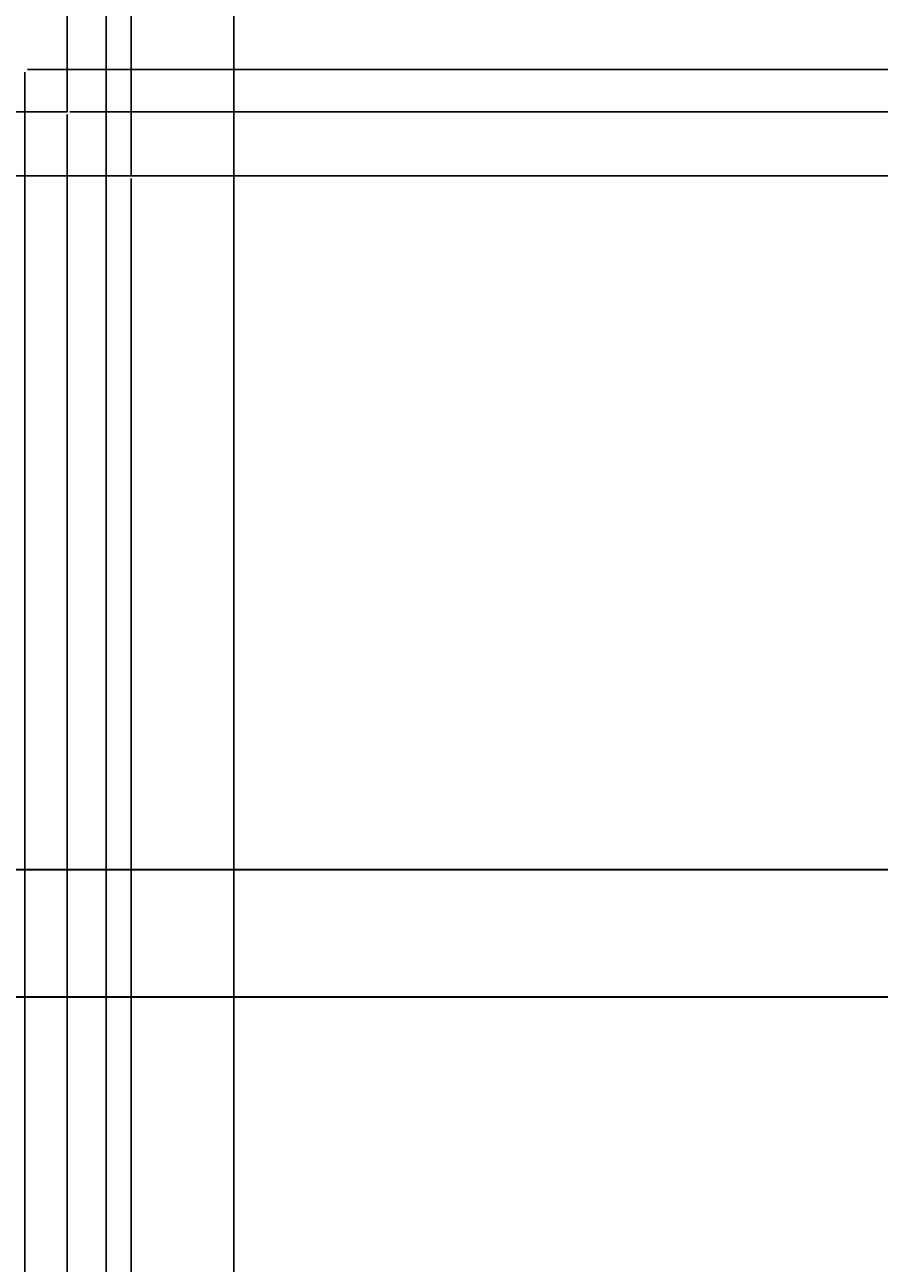
# Model space of a CAD drawing. Units: inches. Extents: x -6 to 289, y -8 to 323.
# Tile 55 of 107: x 166 to 186, y 153 to 182. Entities that reach past the tile are written whole.
import ezdxf

# ---------------------------------------------------------------- set-up
doc = ezdxf.new("R2010")
doc.units = ezdxf.units.IN
doc.header["$MEASUREMENT"] = 0
for name, color, linetype, lineweight in [('A-ANNO-DIMS', 2, 'Continuous', 18), ('A-ELEV', 7, 'Continuous', 35), ('A-GLAZ', 4, 'Continuous', 25)]:
    doc.layers.add(name, color=color, linetype=linetype, lineweight=lineweight)
doc.styles.get("Standard").update_dxf_attribs({"font": 'arial.ttf'})
doc.dimstyles.get("Standard").update_dxf_attribs({"dimtxt": 0.18, "dimasz": 0.18, "dimexe": 0.18, "dimexo": 0.0625, "dimgap": 0.09, "dimtad": 0, "dimtih": 1, "dimtoh": 1, "dimdec": 4, "dimzin": 0, "dimdsep": 46, "dimtxsty": 'Standard', "dimcen": 0.09, "dimadec": 0, "dimazin": 0, "dimtfac": 1, "dimtdec": 4, "dimtofl": 0, "dimtmove": 0, "dimatfit": 3, "dimfxl": 1, "dimtolj": 1, "dimtzin": 0, "dimarcsym": 0})

# ---------------------------------------------------------------- blocks, each defined once
blk = doc.blocks.new('*U4')
for p, q in [((40.5, 46.5), (40.5, 1.5)), ((40.5, 1.5), (21, 1.5))]:
    blk.add_line(p, q)
blk.add_lwpolyline([(0, 0), (0, 48), (42, 48), (42, 0)], close=True)
blk = doc.blocks.new('*D24')
at = {"layer": 'A-ANNO-DIMS', "color": 0, "lineweight": -2, "transparency": 16777216}
for p, q in [((126.946, 178.654), (288.653, 178.654)), ((288.473, 178.474), (288.473, 159.153)), ((288.473, 139.469), (288.473, 158.789)), ((259.226, 139.289), (288.653, 139.289))]:
    blk.add_line(p, q, dxfattribs=at)
at = {"layer": 'A-ANNO-DIMS', "color": 0, "transparency": 16777216}
for points in [[(288.443, 178.474), (288.503, 178.474), (288.473, 178.654)], [(288.443, 139.469), (288.503, 139.469), (288.473, 139.289)]]:
    blk.add_solid(points, dxfattribs=at)
at = {"layer": 'Defpoints', "color": 0, "transparency": 16777216}
for p in [(126.883, 178.654), (288.473, 178.654), (259.164, 139.289)]:
    blk.add_point(p, dxfattribs=at)
at = {"layer": 'A-ANNO-DIMS', "color": 0, "transparency": 16777216, "insert": (288.473, 158.971), "char_height": 0.18, "attachment_point": 5}
blk.add_mtext('\\A1;39.365', dxfattribs=at)
blk = doc.blocks.new('*D25')
at = {"layer": 'A-ANNO-DIMS', "color": 0, "lineweight": -2, "transparency": 16777216}
for p, q in [((126.946, 226.654), (288.653, 226.654)), ((288.473, 226.474), (288.473, 202.836)), ((288.473, 178.834), (288.473, 202.472)), ((126.946, 178.654), (288.653, 178.654))]:
    blk.add_line(p, q, dxfattribs=at)
at = {"layer": 'A-ANNO-DIMS', "color": 0, "transparency": 16777216}
for points in [[(288.443, 226.474), (288.503, 226.474), (288.473, 226.654)], [(288.443, 178.834), (288.503, 178.834), (288.473, 178.654)]]:
    blk.add_solid(points, dxfattribs=at)
at = {"layer": 'Defpoints', "color": 0, "transparency": 16777216}
for p in [(126.883, 226.654), (288.473, 226.654), (126.883, 178.654)]:
    blk.add_point(p, dxfattribs=at)
at = {"layer": 'A-ANNO-DIMS', "color": 0, "transparency": 16777216, "insert": (288.473, 202.654), "char_height": 0.18, "attachment_point": 5}
blk.add_mtext('\\A1;48', dxfattribs=at)
blk = doc.blocks.new('*D32')
at = {"layer": 'A-ANNO-DIMS', "color": 0, "lineweight": -2, "transparency": 16777216}
for p, q in [((147.883, 181.092), (147.883, -8.391)), ((166.383, 181.092), (166.383, -8.391)), ((148.063, -8.211), (156.817, -8.211)), ((166.203, -8.211), (157.449, -8.211))]:
    blk.add_line(p, q, dxfattribs=at)
at = {"layer": 'A-ANNO-DIMS', "color": 0, "transparency": 16777216}
for points in [[(148.063, -8.181), (148.063, -8.241), (147.883, -8.211)], [(166.203, -8.181), (166.203, -8.241), (166.383, -8.211)]]:
    blk.add_solid(points, dxfattribs=at)
at = {"layer": 'Defpoints', "color": 0, "transparency": 16777216}
for p in [(147.883, 181.154), (166.383, 181.154), (166.383, -8.211)]:
    blk.add_point(p, dxfattribs=at)
at = {"layer": 'A-ANNO-DIMS', "color": 0, "transparency": 16777216, "insert": (157.133, -8.211), "char_height": 0.18, "attachment_point": 5}
blk.add_mtext('\\A1;18.5', dxfattribs=at)
blk = doc.blocks.new('*D33')
at = {"layer": 'A-ANNO-DIMS', "color": 0, "lineweight": -2, "transparency": 16777216}
for p, q in [((166.383, 181.092), (166.383, -8.391)), ((167.383, 180.092), (167.383, -8.391)), ((166.563, -8.211), (166.76, -8.211)), ((167.203, -8.211), (167.007, -8.211))]:
    blk.add_line(p, q, dxfattribs=at)
at = {"layer": 'A-ANNO-DIMS', "color": 0, "transparency": 16777216}
for points in [[(166.563, -8.181), (166.563, -8.241), (166.383, -8.211)], [(167.203, -8.181), (167.203, -8.241), (167.383, -8.211)]]:
    blk.add_solid(points, dxfattribs=at)
at = {"layer": 'Defpoints', "color": 0, "transparency": 16777216}
for p in [(166.383, 181.154), (167.383, 180.154), (167.383, -8.211)]:
    blk.add_point(p, dxfattribs=at)
at = {"layer": 'A-ANNO-DIMS', "color": 0, "transparency": 16777216, "insert": (166.883, -8.211), "char_height": 0.18, "attachment_point": 5}
blk.add_mtext('\\A1;1', dxfattribs=at)
blk = doc.blocks.new('*D34')
at = {"layer": 'A-ANNO-DIMS', "color": 0, "lineweight": -2, "transparency": 16777216}
for p, q in [((167.383, 180.092), (167.383, -8.391)), ((168.883, 178.592), (168.883, -8.391)), ((167.563, -8.211), (167.887, -8.211)), ((168.703, -8.211), (168.38, -8.211))]:
    blk.add_line(p, q, dxfattribs=at)
at = {"layer": 'A-ANNO-DIMS', "color": 0, "transparency": 16777216}
for points in [[(167.563, -8.181), (167.563, -8.241), (167.383, -8.211)], [(168.703, -8.181), (168.703, -8.241), (168.883, -8.211)]]:
    blk.add_solid(points, dxfattribs=at)
at = {"layer": 'Defpoints', "color": 0, "transparency": 16777216}
for p in [(167.383, 180.154), (168.883, 178.654), (168.883, -8.211)]:
    blk.add_point(p, dxfattribs=at)
at = {"layer": 'A-ANNO-DIMS', "color": 0, "transparency": 16777216, "insert": (168.133, -8.211), "char_height": 0.18, "attachment_point": 5}
blk.add_mtext('\\A1;1.5', dxfattribs=at)
blk = doc.blocks.new('*D35')
at = {"layer": 'A-ANNO-DIMS', "color": 0, "lineweight": -2, "transparency": 16777216}
for p, q in [((167.446, 180.154), (288.653, 180.154)), ((288.473, 179.974), (288.473, 179.586)), ((288.473, 178.834), (288.473, 179.222)), ((168.946, 178.654), (288.653, 178.654))]:
    blk.add_line(p, q, dxfattribs=at)
at = {"layer": 'A-ANNO-DIMS', "color": 0, "transparency": 16777216}
for points in [[(288.443, 179.974), (288.503, 179.974), (288.473, 180.154)], [(288.443, 178.834), (288.503, 178.834), (288.473, 178.654)]]:
    blk.add_solid(points, dxfattribs=at)
at = {"layer": 'Defpoints', "color": 0, "transparency": 16777216}
for p in [(167.383, 180.154), (288.473, 180.154), (168.883, 178.654)]:
    blk.add_point(p, dxfattribs=at)
at = {"layer": 'A-ANNO-DIMS', "color": 0, "transparency": 16777216, "insert": (288.473, 179.404), "char_height": 0.18, "attachment_point": 5}
blk.add_mtext('\\A1;1.5', dxfattribs=at)
blk = doc.blocks.new('*D36')
at = {"layer": 'A-ANNO-DIMS', "color": 0, "lineweight": -2, "transparency": 16777216}
for p, q in [((166.446, 181.154), (288.653, 181.154)), ((288.473, 180.974), (288.473, 180.834)), ((288.473, 180.334), (288.473, 180.474)), ((167.446, 180.154), (288.653, 180.154))]:
    blk.add_line(p, q, dxfattribs=at)
at = {"layer": 'A-ANNO-DIMS', "color": 0, "transparency": 16777216}
for points in [[(288.443, 180.974), (288.503, 180.974), (288.473, 181.154)], [(288.443, 180.334), (288.503, 180.334), (288.473, 180.154)]]:
    blk.add_solid(points, dxfattribs=at)
at = {"layer": 'Defpoints', "color": 0, "transparency": 16777216}
for p in [(166.383, 181.154), (288.473, 181.154), (167.383, 180.154)]:
    blk.add_point(p, dxfattribs=at)
at = {"layer": 'A-ANNO-DIMS', "color": 0, "transparency": 16777216, "insert": (288.473, 180.654), "char_height": 0.18, "attachment_point": 5}
blk.add_mtext('\\A1;1', dxfattribs=at)
blk = doc.blocks.new('*D37')
at = {"layer": 'A-ANNO-DIMS', "color": 0, "lineweight": -2, "transparency": 16777216}
for p, q in [((166.446, 224.154), (288.653, 224.154)), ((288.473, 223.974), (288.473, 202.836)), ((288.473, 181.334), (288.473, 202.472)), ((166.446, 181.154), (288.653, 181.154))]:
    blk.add_line(p, q, dxfattribs=at)
at = {"layer": 'A-ANNO-DIMS', "color": 0, "transparency": 16777216}
for points in [[(288.443, 223.974), (288.503, 223.974), (288.473, 224.154)], [(288.443, 181.334), (288.503, 181.334), (288.473, 181.154)]]:
    blk.add_solid(points, dxfattribs=at)
at = {"layer": 'Defpoints', "color": 0, "transparency": 16777216}
for p in [(166.383, 224.154), (288.473, 224.154), (166.383, 181.154)]:
    blk.add_point(p, dxfattribs=at)
at = {"layer": 'A-ANNO-DIMS', "color": 0, "transparency": 16777216, "insert": (288.473, 202.654), "char_height": 0.18, "attachment_point": 5}
blk.add_mtext('\\A1;43', dxfattribs=at)
blk = doc.blocks.new('*D77')
at = {"layer": 'A-ANNO-DIMS', "color": 0, "lineweight": -2, "transparency": 16777216}
for p, q in [((164.296, 51.148), (164.296, 322.969)), ((168.296, 51.148), (168.296, 322.969)), ((164.476, 322.789), (166.144, 322.789)), ((168.116, 322.789), (166.448, 322.789))]:
    blk.add_line(p, q, dxfattribs=at)
at = {"layer": 'A-ANNO-DIMS', "color": 0, "transparency": 16777216}
for points in [[(164.476, 322.819), (164.476, 322.759), (164.296, 322.789)], [(168.116, 322.819), (168.116, 322.759), (168.296, 322.789)]]:
    blk.add_solid(points, dxfattribs=at)
at = {"layer": 'Defpoints', "color": 0, "transparency": 16777216}
for p in [(168.296, 322.789), (164.296, 51.085), (168.296, 51.085)]:
    blk.add_point(p, dxfattribs=at)
at = {"layer": 'A-ANNO-DIMS', "color": 0, "transparency": 16777216, "insert": (166.296, 322.789), "char_height": 0.18, "attachment_point": 5}
blk.add_mtext('\\A1;4', dxfattribs=at)
blk = doc.blocks.new('*D78')
at = {"layer": 'A-ANNO-DIMS', "color": 0, "lineweight": -2, "transparency": 16777216}
for p, q in [((168.296, 51.148), (168.296, 322.969)), ((171.296, 51.148), (171.296, 322.969)), ((168.476, 322.789), (169.647, 322.789)), ((171.116, 322.789), (169.945, 322.789))]:
    blk.add_line(p, q, dxfattribs=at)
at = {"layer": 'A-ANNO-DIMS', "color": 0, "transparency": 16777216}
for points in [[(168.476, 322.819), (168.476, 322.759), (168.296, 322.789)], [(171.116, 322.819), (171.116, 322.759), (171.296, 322.789)]]:
    blk.add_solid(points, dxfattribs=at)
at = {"layer": 'Defpoints', "color": 0, "transparency": 16777216}
for p in [(171.296, 322.789), (168.296, 51.085), (171.296, 51.085)]:
    blk.add_point(p, dxfattribs=at)
at = {"layer": 'A-ANNO-DIMS', "color": 0, "transparency": 16777216, "insert": (169.796, 322.789), "char_height": 0.18, "attachment_point": 5}
blk.add_mtext('\\A1;3', dxfattribs=at)
blk = doc.blocks.new('*D79')
at = {"layer": 'A-ANNO-DIMS', "color": 0, "lineweight": -2, "transparency": 16777216}
for p, q in [((171.296, 118.033), (171.296, 322.969)), ((188.292, 116.842), (188.292, 322.969)), ((171.476, 322.789), (179.339, 322.789)), ((188.112, 322.789), (180.249, 322.789))]:
    blk.add_line(p, q, dxfattribs=at)
at = {"layer": 'A-ANNO-DIMS', "color": 0, "transparency": 16777216}
for points in [[(171.476, 322.819), (171.476, 322.759), (171.296, 322.789)], [(188.112, 322.819), (188.112, 322.759), (188.292, 322.789)]]:
    blk.add_solid(points, dxfattribs=at)
at = {"layer": 'Defpoints', "color": 0, "transparency": 16777216}
for p in [(188.292, 322.789), (171.296, 117.971), (188.292, 116.779)]:
    blk.add_point(p, dxfattribs=at)
at = {"layer": 'A-ANNO-DIMS', "color": 0, "transparency": 16777216, "insert": (179.794, 322.789), "char_height": 0.18, "attachment_point": 5}
blk.add_mtext('\\A1;16.996', dxfattribs=at)
blk = doc.blocks.new('*D96')
at = {"layer": 'A-ANNO-DIMS', "color": 0, "lineweight": -2, "transparency": 16777216}
for p, q in [((164.004, 159.411), (164.004, 322.969)), ((200.616, 159.411), (200.616, 322.969)), ((164.184, 322.789), (181.934, 322.789)), ((200.436, 322.789), (182.686, 322.789))]:
    blk.add_line(p, q, dxfattribs=at)
at = {"layer": 'A-ANNO-DIMS', "color": 0, "transparency": 16777216}
for points in [[(164.184, 322.819), (164.184, 322.759), (164.004, 322.789)], [(200.436, 322.819), (200.436, 322.759), (200.616, 322.789)]]:
    blk.add_solid(points, dxfattribs=at)
at = {"layer": 'Defpoints', "color": 0, "transparency": 16777216}
for p in [(200.616, 322.789), (164.004, 159.348), (200.616, 159.348)]:
    blk.add_point(p, dxfattribs=at)
at = {"layer": 'A-ANNO-DIMS', "color": 0, "transparency": 16777216, "insert": (182.31, 322.789), "char_height": 0.18, "attachment_point": 5}
blk.add_mtext('\\A1;36.61', dxfattribs=at)

msp = doc.modelspace()

# ---------------------------------------------------------------- linework, layer by layer
at = {"layer": 'A-ELEV'}
for points in [[(247.1638, 139.2888), (115.1638, 139.2888), (115.1638, 162.3484), (247.1638, 162.3484)], [(244.1638, 142.2888), (118.1638, 142.2888), (118.1638, 159.3484), (244.1638, 159.3484)]]:
    msp.add_lwpolyline(points, close=True, dxfattribs=at)

# ---------------------------------------------------------------- block references
at = {"layer": 'A-GLAZ'}
msp.add_blockref('*U4', (126.8835, 178.654), dxfattribs=at)

# ---------------------------------------------------------------- dimensions: what is measured, and where the dimension line sits
at = {"layer": 'A-ANNO-DIMS'}
for base, p1, p2, override, picture, middle in [((200.6162, 322.7888), (164.0039, 159.3484), (200.6162, 159.3484), {"dimdec": 2, "dimlfac": 1, "dimrnd": 0, "dimzin": 0, "dimdsep": 46, "dimlunit": 2}, '*D96', (182.3101, 322.7888)), ((168.296, 322.7888), (164.296, 51.0851), (168.296, 51.0851), {"dimdec": 0, "dimlfac": 1, "dimrnd": 0, "dimzin": 0, "dimdsep": 46, "dimlunit": 2}, '*D77', (166.296, 322.7888)), ((171.296, 322.7888), (168.296, 51.0851), (171.296, 51.0851), {"dimdec": 0, "dimlfac": 1, "dimrnd": 0, "dimzin": 0, "dimdsep": 46, "dimlunit": 2}, '*D78', (169.796, 322.7888)), ((188.2918, 322.7888), (171.296, 117.9706), (188.2918, 116.7795), {"dimdec": 3, "dimlfac": 1, "dimrnd": 0, "dimzin": 0, "dimdsep": 46, "dimlunit": 2}, '*D79', (179.7939, 322.7888)), ((166.3835, -8.2112), (147.8835, 181.154), (166.3835, 181.154), {"dimdec": 1, "dimlfac": 1, "dimrnd": 0, "dimzin": 0, "dimdsep": 46, "dimlunit": 2}, '*D32', (157.1335, -8.2112)), ((167.3835, -8.2112), (166.3835, 181.154), (167.3835, 180.154), {"dimdec": 0, "dimlfac": 1, "dimrnd": 0, "dimzin": 0, "dimdsep": 46, "dimlunit": 2}, '*D33', (166.8835, -8.2112)), ((168.8835, -8.2112), (167.3835, 180.154), (168.8835, 178.654), {"dimdec": 1, "dimlfac": 1, "dimrnd": 0, "dimzin": 0, "dimdsep": 46, "dimlunit": 2}, '*D34', (168.1335, -8.2112))]:
    dim = msp.add_linear_dim(base=base, p1=p1, p2=p2, dimstyle='Standard', override=override, dxfattribs=at)
    dim.commit()
    dim.dimension.update_dxf_attribs({"geometry": picture, "text_midpoint": middle})
for base, p1, p2, override, picture, middle in [((288.4733, 226.654), (126.8835, 178.654), (126.8835, 226.654), {"dimdec": 0, "dimlfac": 1, "dimrnd": 0, "dimzin": 0, "dimdsep": 46, "dimlunit": 2}, '*D25', (288.4733, 202.654)), ((288.4733, 224.154), (166.3835, 181.154), (166.3835, 224.154), {"dimdec": 0, "dimlfac": 1, "dimrnd": 0, "dimzin": 0, "dimdsep": 46, "dimlunit": 2}, '*D37', (288.4733, 202.654)), ((288.4733, 181.154), (167.3835, 180.154), (166.3835, 181.154), {"dimdec": 0, "dimlfac": 1, "dimrnd": 0, "dimzin": 0, "dimdsep": 46, "dimlunit": 2}, '*D36', (288.4733, 180.654)), ((288.4733, 180.154), (168.8835, 178.654), (167.3835, 180.154), {"dimdec": 1, "dimlfac": 1, "dimrnd": 0, "dimzin": 0, "dimdsep": 46, "dimlunit": 2}, '*D35', (288.4733, 179.404)), ((288.4733, 178.654), (259.1638, 139.2888), (126.8835, 178.654), {"dimdec": 3, "dimlfac": 1, "dimrnd": 0, "dimzin": 0, "dimdsep": 46, "dimlunit": 2}, '*D24', (288.4733, 158.9714))]:
    dim = msp.add_linear_dim(base=base, p1=p1, p2=p2, angle=90, dimstyle='Standard', override=override, dxfattribs=at)
    dim.commit()
    dim.dimension.update_dxf_attribs({"geometry": picture, "text_midpoint": middle})

doc.saveas('drawing.dxf')
